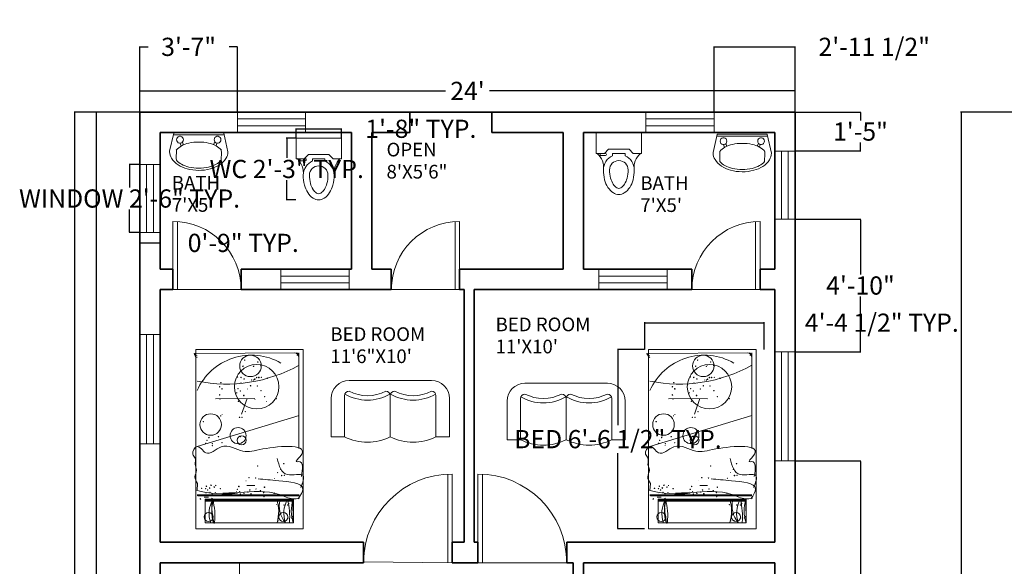
# Model space of a CAD drawing. Units: inches. Extents: x 125 to 976, y 231 to 853.
# Tile 11 of 16: x 125 to 557, y 613 to 853. Entities that reach past the tile are written whole.
import ezdxf

# ---------------------------------------------------------------- set-up
doc = ezdxf.new("R2010")
doc.units = ezdxf.units.IN
doc.header["$MEASUREMENT"] = 0
for name, color, linetype, lineweight in [('A-ANNO-DIMS', 2, 'Continuous', 18), ('A-AREA-IDEN', 7, 'Continuous', 18), ('A-DOOR', 3, 'Continuous', 18), ('A-FLOR-CASE', 32, 'Continuous', 18), ('A-FLOR-FIXT', 9, 'Continuous', 18), ('A-GLAZ', 4, 'Continuous', 18), ('A-WALL', 7, 'Continuous', 35), ('Furniture', 8, 'Continuous', 15)]:
    doc.layers.add(name, color=color, linetype=linetype, lineweight=lineweight)
doc.styles.get("Standard").update_dxf_attribs({"font": 'italic8.shx'})
doc.dimstyles.get("Standard").update_dxf_attribs({"dimtxt": 8, "dimasz": 0.18, "dimexe": 0.18, "dimexo": 0.0625, "dimgap": 0.09, "dimtad": 0, "dimtih": 1, "dimtoh": 1, "dimdec": 4, "dimzin": 0, "dimdsep": 46, "dimlunit": 3, "dimtxsty": 'Standard', "dimcen": 0.09, "dimclrt": 4, "dimadec": 0, "dimazin": 0, "dimtfac": 1, "dimtdec": 4, "dimtofl": 0, "dimtmove": 0, "dimatfit": 3, "dimfxl": 1, "dimtolj": 1, "dimtzin": 0, "dimarcsym": 0})

# ---------------------------------------------------------------- blocks, each defined once
blk = doc.blocks.new('*D3')
at = {"layer": 'A-ANNO-DIMS', "color": 0, "lineweight": -2, "transparency": 16777216}
for p, q in [((177.58, 812.17), (177.58, 821.62)), ((177.76, 821.44), (311.97, 821.44)), ((465.4, 821.44), (331.19, 821.44)), ((465.58, 812.17), (465.58, 821.62))]:
    blk.add_line(p, q, dxfattribs=at)
at = {"layer": 'A-ANNO-DIMS', "color": 0, "transparency": 16777216}
for points in [[(177.76, 821.47), (177.76, 821.41), (177.58, 821.44)], [(465.4, 821.47), (465.4, 821.41), (465.58, 821.44)]]:
    blk.add_solid(points, dxfattribs=at)
at = {"layer": 'Defpoints', "color": 0, "transparency": 16777216}
for p in [(465.58, 821.44), (177.58, 812.1), (465.58, 812.1)]:
    blk.add_point(p, dxfattribs=at)
at = {"layer": 'A-ANNO-DIMS', "color": 0, "transparency": 16777216, "insert": (321.58, 821.44), "char_height": 8, "attachment_point": 5}
blk.add_mtext("\\A1;24'", dxfattribs=at)
blk = doc.blocks.new('*D4')
at = {"layer": 'A-ANNO-DIMS', "color": 0, "lineweight": -2, "transparency": 16777216}
for p, q in [((177.52, 812.1), (158.26, 812.1)), ((158.44, 811.92), (158.44, 546.96)), ((158.44, 272.28), (158.44, 537.25)), ((177.52, 272.1), (158.26, 272.1))]:
    blk.add_line(p, q, dxfattribs=at)
at = {"layer": 'A-ANNO-DIMS', "color": 0, "transparency": 16777216}
for points in [[(158.41, 811.92), (158.47, 811.92), (158.44, 812.1)], [(158.41, 272.28), (158.47, 272.28), (158.44, 272.1)]]:
    blk.add_solid(points, dxfattribs=at)
at = {"layer": 'Defpoints', "color": 0, "transparency": 16777216}
for p in [(177.58, 812.1), (158.44, 272.1), (177.58, 272.1)]:
    blk.add_point(p, dxfattribs=at)
at = {"layer": 'A-ANNO-DIMS', "color": 0, "transparency": 16777216, "insert": (158.44, 542.1), "char_height": 8, "attachment_point": 5}
blk.add_mtext("\\A1;45'", dxfattribs=at)
blk = doc.blocks.new('BED-SINGLE')
for p, q in [((1.36, 0), (1.36, 78.74)), ((1.36, 78.74), (48.6, 78.74)), ((48.6, 78.74), (48.6, 0)), ((45.57, 77.25), (0.68, 77.02)), ((46.62, 76.32), (45.83, 76.32)), ((46.75, 35.25), (46.75, 77.26)), ((46.75, 35.25), (46.75, 75.28)), ((10.09, 57.07), (27.33, 57.29)), ((21.53, 50.36), (23.91, 57.3)), ((46.77, 49.81), (2, 36.21)), ((46.74, 50.11), (46.74, 35.53)), ((2.2, 19.89), (1.98, 16.84)), ((23.9, 19.06), (27.33, 19.06)), ((46.77, 14.92), (2, 14.9)), ((46.77, 14.62), (2, 14.6)), ((46.75, 14.47), (2.3, 14.45)), ((5.12, 13.84), (6.96, 13.84)), ((44.11, 12.79), (5.52, 12.79)), ((44.11, 12.66), (5.52, 12.66)), ((44.11, 12.36), (5.52, 12.36)), ((44.11, 12.07), (5.52, 12.07)), ((5.56, 2.64), (5.56, 12.97)), ((5.56, 12.97), (44.32, 12.97)), ((44.26, 2.65), (44.11, 12.79)), ((44.32, 12.97), (44.32, 2.64)), ((44.32, 2.64), (5.56, 2.64)), ((1.36, 0), (48.6, 0))]:
    blk.add_line(p, q)
for centre, radius in [((25.44, 71.55), 4.72), ((22.93, 74.08), 0.0787), ((28.17, 62.4), 9.76), ((22.09, 71.4), 0.118), ((26.78, 71.35), 0.118), ((27.34, 71.86), 0.0394), ((28.65, 73.29), 0.118), ((30.02, 71.69), 0.118), ((19.72, 66.71), 0.118), ((21.26, 66.47), 0.118), ((22.64, 65.78), 0.118), ((25.97, 65.38), 0.0394), ((26.83, 65.34), 0.118), ((27.33, 65.73), 0.118), ((28.16, 66.42), 0.118), ((29.11, 66.45), 0.118), ((30.23, 66.51), 0.0787), ((32.84, 66.14), 0.118), ((11.89, 62.39), 0.118), ((12.45, 64.21), 0.118), ((12.91, 61.47), 0.118), ((19.93, 61.53), 0.0787), ((21.3, 64.04), 0.0787), ((24.15, 61.41), 0.0394), ((25.46, 62.84), 0.118), ((28.4, 62.67), 0.0787), ((30.08, 60.69), 0.118), ((11.89, 58.82), 0.118), ((12.09, 56.97), 0.0787), ((19.37, 59.72), 0.0787), ((22.48, 58.54), 0.118), ((27.41, 56.76), 0.0394), ((31.66, 58.02), 0.0787), ((36.84, 57.2), 0.0787), ((20.18, 56), 0.118), ((32.59, 55.94), 0.0394), ((7.95, 45.79), 4.72), ((12.36, 49.61), 0.0787), ((12.97, 50.24), 0.0394), ((20.64, 48.94), 0.118), ((21.75, 49), 0.0787), ((23.12, 51.5), 0.0787), ((4.72, 47.06), 0.118), ((20, 40.91), 3.54), ((7.15, 40.05), 0.118), ((11.34, 40.44), 0.118), ((21.58, 38.87), 1.97), ((5.78, 37.54), 0.118), ((6.3, 38.84), 0.0787), ((8.67, 36.51), 0.0394), ((8.72, 37.38), 0.0787), ((12.92, 37.77), 0.0787), ((19.76, 37.58), 0.0394), ((28.63, 27.54), 0.0787), ((38.69, 26.11), 0.118), ((40.06, 28.61), 0.118), ((24.77, 22.46), 0.118), ((27.72, 22.29), 0.0787), ((36.01, 22.18), 0.0394), ((37.38, 24.68), 0.0394), ((39.15, 23.37), 0.118), ((40.26, 23.43), 0.0787), ((3.99, 17.75), 0.118), ((5.75, 17.64), 0.0787), ((6.1, 18.69), 0.118), ((7.26, 18.11), 0.0394), ((7.48, 17.87), 0.118), ((8.13, 19.13), 0.118), ((9.51, 18.3), 0.118), ((10.16, 19), 0.0787), ((12.17, 17.6), 0.118), ((19.68, 17.32), 0.118), ((20.33, 18.58), 0.118), ((23.46, 21.04), 0.0394), ((27.92, 17.51), 0.0787), ((31.59, 18.26), 0.118), ((3.44, 13.12), 0.118), ((5.89, 15.61), 0.0394), ((6.65, 17.04), 0.118), ((7.14, 14.65), 0.0394), ((7.68, 16.02), 0.0787), ((8.57, 13.26), 0.118), ((8.58, 15.39), 0.118), ((9.94, 15.76), 0.118), ((11.85, 14.52), 0.118), ((19.22, 16.39), 0.0394), ((20.71, 16.3), 0.0787), ((22.61, 15.56), 0.118), ((24.29, 16.17), 0.118), ((25.12, 17), 0.118), ((25.67, 15.35), 0.118), ((29.81, 16.72), 0.118), ((31.19, 15.9), 0.118), ((31.38, 14.05), 0.0787), ((35.87, 15.62), 0.118), ((36.87, 10.58), 0.0394), ((40.18, 10.43), 0.118), ((41.76, 10.43), 0.118), ((42.23, 11.05), 0.118), ((7.01, 5.19), 1.97), ((37.65, 4.55), 0.0394), ((39.85, 5.18), 1.97), ((41.9, 4.7), 0.0787), ((43.48, 4.7), 0.0787), ((43.95, 5.33), 0.0787), ((37.65, 3.45), 0.0394), ((39.23, 3.45), 0.0394), ((39.7, 4.08), 0.0394)]:
    blk.add_circle(centre, radius)
for centre, radius, start, end in [((1.8, 77.16), 1.13, 187.0311, 279.2977), ((2.15, 76.26), 1.02, 131.9337, 260.5378), ((25.86, 50.2), 26.08, 60.1506, 156.1931), ((44.78, 75.28), 1.97, 0, 90), ((45.57, 76.07), 1.18, 0, 90), ((14.92, 129.11), 65.53, 258.633, 299.0775), ((14.39, 67.77), 52.46, 255.8437, 275.7821), ((19.25, 6.76), 12.01, 149.8072, 199.9256), ((25.9, 7.71), 17.5, 163.1329, 196.7593), ((39.3, 10.2), 30.85, 175.6161, 194.8863), ((-19.02, 5.5), 28.83, 354.7074, 14.6885), ((19.98, 7.67), 17.85, 343.6634, 17.1743), ((49.46, 10.01), 11.36, 165.8396, 220.337), ((52.09, 6.75), 12.01, 149.8072, 199.9256), ((13.83, 5.48), 28.83, 354.7074, 14.6885), ((59.92, 7.95), 16.53, 163.0006, 198.6759)]:
    blk.add_arc(centre, radius, start, end)
for points, knots in [([(47.83, 23.01), (48.39, 26.23), (49.02, 29.87), (44.73, 29.28), (54.44, 37.77), (31.08, 35.83), (22.32, 32.61), (13.25, 38.92), (6.29, 30.55), (2.31, 38.17), (-0.92, 33.01), (1.74, 30.96), (0.68, 28.27), (2.31, 25.67), (0.37, 22.75), (1.58, 20.86), (2.2, 19.89)], [0, 0, 0, 0, 6.608381, 7.436978, 10.160479, 26.82811, 35.651646, 45.441607, 52.697614, 57.347481, 61.162366, 63.231685, 65.951856, 68.505046, 71.545852, 74.730692, 74.730692, 74.730692, 74.730692]), ([(47.57, 18.18), (48.41, 20.34), (50.37, 25.33), (39.55, 21.84), (38.02, 27.69), (37.18, 30.9)], [0, 0, 0, 0, 5.247261, 12.129135, 20.530793, 20.530793, 20.530793, 20.530793]), ([(46.4, 13.16), (47.43, 14.71), (50.88, 19.94), (37.54, 21.11), (31.56, 21.67), (28.88, 21.92)], [0, 0, 0, 0, 4.712342, 15.867179, 24.91455, 24.91455, 24.91455, 24.91455]), ([(13.24, 15.66), (15.6, 15.7), (23.87, 15.87), (34.62, 17.37), (42.93, 12.79), (46.01, 13.25), (47.01, 13.4)], [0, 0, 0, 0, 7.121262, 24.909491, 31.123221, 34.101394, 34.101394, 34.101394, 34.101394])]:
    blk.add_open_spline(points, degree=3, knots=knots)
for p in [(21.03, 60.57), (21.03, 40.49), (21.03, 15.28)]:
    blk.add_point(p)
blk = doc.blocks.new('WC')
for p, q in [((0, 27.17), (19.92, 27.17)), ((0, 27.17), (0, 18.11)), ((19.92, 27.17), (19.92, 18.11)), ((0, 18.11), (3.62, 18.11)), ((1.81, 18.11), (1.81, 17.21)), ((5.43, 19.92), (3.62, 18.11)), ((4.07, 18.11), (3.62, 18.11)), ((5.43, 19.92), (14.48, 19.92)), ((12.67, 18.11), (7.24, 18.11)), ((7.24, 18.11), (7.24, 17.09)), ((12.67, 18.11), (12.67, 17.09)), ((14.48, 19.92), (16.3, 18.11)), ((19.92, 18.11), (16.3, 18.11)), ((1.81, 17.21), (4.07, 17.21))]:
    blk.add_line(p, q)
for centre, radius, start, end in [((-4.9, 11.97), 8.15, 352.2011, 48.911), ((4.07, 17.66), 0.453, 270, 90), ((24.82, 11.97), 8.15, 131.089, 187.7989), ((9.96, 10.87), 6.79, 113.5782, 180), ((9.96, 10.87), 4.07, 0, 180), ((9.96, 10.87), 6.79, 0, 66.4218), ((20.49, 10.87), 17.33, 180, 194.5143), ((20.49, 10.87), 14.61, 180, 194.5142), ((-0.58, 10.87), 14.61, 345.4858, 360), ((-0.58, 10.87), 17.33, 345.4857, 360), ((15.3, 9.52), 11.96, 194.5143, 212.0054), ((15.3, 9.52), 9.24, 194.5143, 212.0054), ((12.02, 7.47), 5.38, 212.0054, 236.4659), ((7.9, 7.47), 5.38, 303.5341, 327.9946), ((4.62, 9.52), 9.24, 327.9946, 345.4857), ((4.62, 9.52), 11.96, 327.9946, 345.4857), ((12.02, 7.47), 8.09, 212.0054, 236.4659), ((9.96, 4.37), 4.36, 236.4659, 270), ((9.96, 4.37), 1.65, 236.466, 270), ((9.96, 4.37), 1.65, 270, 303.534), ((9.96, 4.37), 4.36, 270, 303.5341), ((7.9, 7.47), 8.09, 303.5341, 327.9946)]:
    blk.add_arc(centre, radius, start, end)
blk = doc.blocks.new('BASIN')
for p, q in [((0.01, 8.4), (1.8, 16.33)), ((1.8, 16.54), (23.8, 16.54)), ((1.8, 16.13), (1.8, 16.54)), ((23.8, 15.65), (1.8, 15.65)), ((3.17, 14), (3.08, 13.48)), ((3.08, 13.48), (3.17, 12.95)), ((3.42, 14.46), (3.17, 14)), ((3.81, 14.8), (3.42, 14.46)), ((4.29, 14.98), (3.81, 14.8)), ((4.81, 14.98), (4.29, 14.98)), ((5.29, 14.8), (4.81, 14.98)), ((5.68, 14.46), (5.29, 14.8)), ((5.93, 14), (5.68, 14.46)), ((6.02, 13.48), (5.93, 14)), ((5.93, 12.95), (6.02, 13.48)), ((19.66, 14), (19.58, 13.48)), ((19.58, 13.48), (19.66, 12.95)), ((19.92, 14.46), (19.66, 14)), ((20.31, 14.8), (19.92, 14.46)), ((20.79, 14.98), (20.31, 14.8)), ((21.3, 14.98), (20.79, 14.98)), ((21.79, 14.8), (21.3, 14.98)), ((22.18, 14.46), (21.79, 14.8)), ((22.43, 14), (22.18, 14.46)), ((22.52, 13.48), (22.43, 14)), ((22.43, 12.95), (22.52, 13.48)), ((23.8, 16.54), (23.8, 16.13)), ((25.59, 8.23), (23.8, 16.33)), ((2.96, 8.83), (2.87, 5.21)), ((2.97, 8.99), (2.96, 8.98)), ((2.96, 8.98), (2.96, 8.97)), ((2.96, 8.97), (2.96, 8.96)), ((2.96, 8.83), (2.96, 8.96)), ((3.07, 9.08), (2.97, 8.99)), ((3.17, 12.95), (3.42, 12.49)), ((3.42, 12.49), (3.81, 12.15)), ((3.81, 12.15), (4.29, 11.97)), ((4.29, 11.97), (4.81, 11.97)), ((4.57, 11.96), (5.02, 10.67)), ((4.81, 11.97), (5.29, 12.15)), ((5.29, 12.15), (5.68, 12.49)), ((5.63, 12.45), (6.09, 11.17)), ((5.68, 12.49), (5.93, 12.95)), ((19.87, 12.63), (19.34, 11.26)), ((19.66, 12.95), (19.92, 12.49)), ((19.92, 12.49), (20.31, 12.15)), ((20.31, 12.15), (20.79, 11.97)), ((20.73, 11.97), (20.41, 10.75)), ((20.79, 11.97), (21.3, 11.97)), ((21.3, 11.97), (21.79, 12.15)), ((21.79, 12.15), (22.18, 12.49)), ((22.18, 12.49), (22.43, 12.95)), ((22.76, 8.08), (22.65, 8.8)), ((2.87, 5.21), (3, 4.47)), ((22.54, 4.2), (22.57, 4.35)), ((22.6, 4.46), (22.76, 8.08)), ((3.05, 4.25), (3.05, 4.25))]:
    blk.add_line(p, q)
for centre, radius, start, end in [((8.91, 3.9), 7.83, 118.2302, 139.6822), ((11.35, -0.82), 13.14, 102.6999, 117.8694), ((12.88, -8.38), 20.85, 90.2298, 102.2344), ((12.72, -8.38), 20.85, 77.7656, 89.7702), ((14.25, -0.82), 13.14, 62.1306, 77.3001), ((16.68, 3.89), 7.83, 39.3299, 61.7657), ((5.18, 8.21), 5.18, 177.9266, 179.8113), ((5.16, 8.15), 5.16, 179.1785, 213.1413), ((8.98, 10.54), 9.66, 212.6461, 237.0936), ((8.91, 9.59), 7.83, 220.8964, 241.7723), ((16.69, 9.59), 7.83, 298.2281, 319.1983), ((16.64, 10.51), 9.66, 302.4413, 326.8887), ((20.44, 8.09), 5.16, 326.4084, 0.3713), ((20.42, 8.14), 5.18, 359.7541, 0.9471), ((11.42, 14.45), 14.27, 237.383, 254.6821), ((11.35, 14.31), 13.14, 242.1306, 257.3001), ((12.95, 20.75), 20.75, 255.1956, 269.4863), ((12.88, 21.87), 20.85, 257.7656, 269.7702), ((12.76, 20.75), 20.75, 270.0316, 284.3223), ((12.72, 21.87), 20.85, 270.2298, 282.2344), ((14.25, 14.31), 13.14, 282.6999, 297.8694), ((14.23, 14.44), 14.27, 284.841, 302.14)]:
    blk.add_arc(centre, radius, start, end)
blk = doc.blocks.new('LOVESEAT')
for p, q in [((44.1, 27.17, -27), (7.88, 27.17, -27)), ((0, 19.29, -27), (0, 2.36, -27)), ((5.91, 20.47, -27), (5.91, 2.36, -27)), ((5.91, 2.36, -27), (5.91, 20.47, -27)), ((5.91, 20.47, -27), (5.91, 2.36, -27)), ((25.99, 2.36, -27), (25.99, 20.47, -27)), ((25.99, 20.47, -27), (25.99, 2.36, -27)), ((46.07, 20.47, -27), (46.07, 2.36, -27)), ((51.97, 2.36, -27), (51.97, 19.29, -27)), ((0, 2.36, -27), (5.91, 2.36, -27)), ((51.97, 2.36, -27), (46.07, 2.36, -27))]:
    blk.add_line(p, q)
for centre, radius, start, end in [((7.88, 19.29, -27), 7.87, 90, 180), ((44.1, 19.29, -27), 7.87, 0, 90), ((7.88, 20.47, -27), 1.97, 90, 180), ((15.95, 38, -27), 17.53, 242.5861, 297.4139), ((24.02, 20.47, -27), 1.97, 0, 90), ((27.96, 20.47, -27), 1.97, 90, 180), ((36.03, 38, -27), 17.53, 242.5861, 297.4139), ((44.1, 20.47, -27), 1.97, 0, 90), ((15.95, 38, -27), 19.5, 239.4911, 300.5089), ((36.03, 38, -27), 19.5, 239.4911, 300.5089), ((15.95, 22.51, -27), 22.51, 243.519, 296.481), ((36.03, 22.51, -27), 22.51, 243.519, 296.481)]:
    blk.add_arc(centre, radius, start, end)
blk = doc.blocks.new('WINDOW-48IN')
for p, q in [((0, 0), (0, 48)), ((0, 48), (9, 48)), ((3, 0), (3, 48)), ((6, 0), (6, 48)), ((9, 48), (9, 0)), ((9, 0), (0, 0))]:
    blk.add_line(p, q)
blk = doc.blocks.new('WINDOW-30IN')
for p, q in [((0, 0), (0, 9)), ((0, 9), (30, 9)), ((30, 9), (30, 0)), ((30, 6), (0, 6)), ((30, 3), (0, 3)), ((30, 0), (0, 0))]:
    blk.add_line(p, q)
blk = doc.blocks.new('DOOR-39IN-LH')
for p, q in [((-2, 0), (-2, 38.95)), ((0, 0), (0, 39)), ((-39, 0.34), (0, 0))]:
    blk.add_line(p, q)
blk.add_arc((0, 0), 39, 90, 179.5065)
blk = doc.blocks.new('DOOR-39IN-RH')
for p, q in [((0, 39), (0, 0)), ((2, 38.95), (2, 0)), ((0, 0), (39, 0))]:
    blk.add_line(p, q)
blk.add_arc((0, 0), 39, 0, 90)
blk = doc.blocks.new('DOOR-30IN')
for p, q in [((-2, 29.93), (-2, 0)), ((0, 30), (0, 0)), ((0, 0), (-30, 0))]:
    blk.add_line(p, q)
blk.add_arc((0, 0), 30, 90, 180)
blk = doc.blocks.new('*D26')
at = {"layer": 'A-ANNO-DIMS', "color": 0, "lineweight": -2, "transparency": 16777216}
for p, q in [((177.52, 789.16), (172.9, 789.16)), ((173.08, 788.98), (173.08, 779.01)), ((173.08, 759.34), (173.08, 769.3)), ((177.52, 759.16), (172.9, 759.16))]:
    blk.add_line(p, q, dxfattribs=at)
at = {"layer": 'A-ANNO-DIMS', "color": 0, "transparency": 16777216}
for points in [[(173.05, 788.98), (173.11, 788.98), (173.08, 789.16)], [(173.05, 759.34), (173.11, 759.34), (173.08, 759.16)]]:
    blk.add_solid(points, dxfattribs=at)
at = {"layer": 'Defpoints', "color": 0, "transparency": 16777216}
for p in [(177.58, 789.16), (173.08, 759.16), (177.58, 759.16)]:
    blk.add_point(p, dxfattribs=at)
at = {"layer": 'A-ANNO-DIMS', "color": 4, "transparency": 16777216, "insert": (173.08, 774.16), "char_height": 8, "attachment_point": 5}
blk.add_mtext('\\A1;WINDOW 2\'-6" TYP.', dxfattribs=at)
blk = doc.blocks.new('*D27')
at = {"layer": 'A-ANNO-DIMS', "color": 0, "lineweight": -2, "transparency": 16777216}
for p, q in [((177.58, 759.09), (177.58, 754.48)), ((186.58, 759.09), (186.58, 754.48)), ((177.76, 754.66), (186.4, 754.66)), ((186.58, 754.66), (186.76, 754.66))]:
    blk.add_line(p, q, dxfattribs=at)
at = {"layer": 'A-ANNO-DIMS', "color": 0, "transparency": 16777216}
for points in [[(177.76, 754.69), (177.76, 754.63), (177.58, 754.66)], [(186.4, 754.69), (186.4, 754.63), (186.58, 754.66)]]:
    blk.add_solid(points, dxfattribs=at)
at = {"layer": 'Defpoints', "color": 0, "transparency": 16777216}
for p in [(177.58, 759.16), (186.58, 759.16), (186.58, 754.66)]:
    blk.add_point(p, dxfattribs=at)
at = {"layer": 'A-ANNO-DIMS', "color": 4, "transparency": 16777216, "insert": (223.04, 754.66), "char_height": 8, "attachment_point": 5}
blk.add_mtext('\\A1;0\'-9" TYP.', dxfattribs=at)
blk = doc.blocks.new('*D30')
at = {"layer": 'A-ANNO-DIMS', "color": 0, "lineweight": -2, "transparency": 16777216}
for p, q in [((399.43, 707.79), (387.5, 707.79)), ((387.68, 707.61), (387.68, 674.6)), ((387.68, 629.23), (387.68, 662.23)), ((399.43, 629.05), (387.5, 629.05))]:
    blk.add_line(p, q, dxfattribs=at)
at = {"layer": 'A-ANNO-DIMS', "color": 0, "transparency": 16777216}
for points in [[(387.65, 707.61), (387.71, 707.61), (387.68, 707.79)], [(387.65, 629.23), (387.71, 629.23), (387.68, 629.05)]]:
    blk.add_solid(points, dxfattribs=at)
at = {"layer": 'Defpoints', "color": 0, "transparency": 16777216}
for p in [(387.68, 707.79), (399.49, 707.79), (399.49, 629.05)]:
    blk.add_point(p, dxfattribs=at)
at = {"layer": 'A-ANNO-DIMS', "color": 4, "transparency": 16777216, "insert": (387.68, 668.42), "char_height": 8, "attachment_point": 5}
blk.add_mtext('\\A1;BED 6\'-6 1/2" TYP.', dxfattribs=at)
blk = doc.blocks.new('*D31')
at = {"layer": 'A-ANNO-DIMS', "color": 0, "lineweight": -2, "transparency": 16777216}
for p, q in [((399.49, 707.85), (399.49, 719.78)), ((399.67, 719.6), (451.78, 719.6)), ((451.96, 707.85), (451.96, 719.78)), ((451.96, 719.6), (452.14, 719.6))]:
    blk.add_line(p, q, dxfattribs=at)
at = {"layer": 'A-ANNO-DIMS', "color": 0, "transparency": 16777216}
for points in [[(399.67, 719.63), (399.67, 719.57), (399.49, 719.6)], [(451.78, 719.63), (451.78, 719.57), (451.96, 719.6)]]:
    blk.add_solid(points, dxfattribs=at)
at = {"layer": 'Defpoints', "color": 0, "transparency": 16777216}
for p in [(451.96, 719.6), (399.49, 707.79), (451.96, 707.79)]:
    blk.add_point(p, dxfattribs=at)
at = {"layer": 'A-ANNO-DIMS', "color": 4, "transparency": 16777216, "insert": (503.66, 719.6), "char_height": 8, "attachment_point": 5}
blk.add_mtext('\\A1;4\'-4 1/2" TYP.', dxfattribs=at)
blk = doc.blocks.new('*D32')
at = {"layer": 'A-ANNO-DIMS', "color": 0, "lineweight": -2, "transparency": 16777216}
for p, q in [((246.17, 800.72), (241.97, 800.72)), ((242.15, 800.54), (242.15, 791.99)), ((242.15, 773.74), (242.15, 782.29)), ((246.17, 773.56), (241.97, 773.56))]:
    blk.add_line(p, q, dxfattribs=at)
at = {"layer": 'A-ANNO-DIMS', "color": 0, "transparency": 16777216}
for points in [[(242.12, 800.54), (242.18, 800.54), (242.15, 800.72)], [(242.12, 773.74), (242.18, 773.74), (242.15, 773.56)]]:
    blk.add_solid(points, dxfattribs=at)
at = {"layer": 'Defpoints', "color": 0, "transparency": 16777216}
for p in [(242.15, 800.72), (246.23, 800.72), (246.23, 773.56)]:
    blk.add_point(p, dxfattribs=at)
at = {"layer": 'A-ANNO-DIMS', "color": 4, "transparency": 16777216, "insert": (242.15, 787.14), "char_height": 8, "attachment_point": 5}
blk.add_mtext('\\A1;WC 2\'-3" TYP.', dxfattribs=at)
blk = doc.blocks.new('*D33')
at = {"layer": 'A-ANNO-DIMS', "color": 0, "lineweight": -2, "transparency": 16777216}
for p, q in [((246.23, 800.79), (246.23, 804.98)), ((266.15, 800.79), (266.15, 804.98)), ((246.41, 804.8), (265.97, 804.8)), ((266.15, 804.8), (266.33, 804.8))]:
    blk.add_line(p, q, dxfattribs=at)
at = {"layer": 'A-ANNO-DIMS', "color": 0, "transparency": 16777216}
for points in [[(246.41, 804.83), (246.41, 804.77), (246.23, 804.8)], [(265.97, 804.83), (265.97, 804.77), (266.15, 804.8)]]:
    blk.add_solid(points, dxfattribs=at)
at = {"layer": 'Defpoints', "color": 0, "transparency": 16777216}
for p in [(246.23, 800.72), (266.15, 804.8), (266.15, 800.72)]:
    blk.add_point(p, dxfattribs=at)
at = {"layer": 'A-ANNO-DIMS', "color": 4, "transparency": 16777216, "insert": (301.09, 804.8), "char_height": 8, "attachment_point": 5}
blk.add_mtext('\\A1;1\'-8" TYP.', dxfattribs=at)
blk = doc.blocks.new('*D56')
at = {"layer": 'A-ANNO-DIMS', "color": 0, "lineweight": -2, "transparency": 16777216}
for p, q in [((177.52, 812.1), (148.7, 812.1)), ((148.88, 811.92), (148.88, 575.46)), ((148.88, 329.28), (148.88, 565.75)), ((186.52, 329.1), (148.7, 329.1))]:
    blk.add_line(p, q, dxfattribs=at)
at = {"layer": 'A-ANNO-DIMS', "color": 0, "transparency": 16777216}
for points in [[(148.85, 811.92), (148.91, 811.92), (148.88, 812.1)], [(148.85, 329.28), (148.91, 329.28), (148.88, 329.1)]]:
    blk.add_solid(points, dxfattribs=at)
at = {"layer": 'Defpoints', "color": 0, "transparency": 16777216}
for p in [(148.88, 812.1), (177.58, 812.1), (186.58, 329.1)]:
    blk.add_point(p, dxfattribs=at)
at = {"layer": 'A-ANNO-DIMS', "color": 4, "transparency": 16777216, "insert": (148.88, 570.6), "char_height": 8, "attachment_point": 5}
blk.add_mtext('\\A1;40\'-3"', dxfattribs=at)
blk = doc.blocks.new('*D57')
at = {"layer": 'A-ANNO-DIMS', "color": 0, "lineweight": -2, "transparency": 16777216}
for p, q in [((567.13, 812.1), (538.31, 812.1)), ((538.49, 811.92), (538.49, 575.46)), ((538.49, 329.28), (538.49, 565.75)), ((576.13, 329.1), (538.31, 329.1))]:
    blk.add_line(p, q, dxfattribs=at)
at = {"layer": 'A-ANNO-DIMS', "color": 0, "transparency": 16777216}
for points in [[(538.46, 811.92), (538.52, 811.92), (538.49, 812.1)], [(538.46, 329.28), (538.52, 329.28), (538.49, 329.1)]]:
    blk.add_solid(points, dxfattribs=at)
at = {"layer": 'Defpoints', "color": 0, "transparency": 16777216}
for p in [(538.49, 812.1), (567.19, 812.1), (576.19, 329.1)]:
    blk.add_point(p, dxfattribs=at)
at = {"layer": 'A-ANNO-DIMS', "color": 4, "transparency": 16777216, "insert": (538.49, 570.6), "char_height": 8, "attachment_point": 5}
blk.add_mtext('\\A1;40\'-3"', dxfattribs=at)
blk = doc.blocks.new('*D64')
at = {"layer": 'A-ANNO-DIMS', "color": 0, "lineweight": -2, "transparency": 16777216}
for p, q in [((465.64, 658.83), (494.46, 658.83)), ((494.28, 658.65), (494.28, 561.16)), ((494.28, 451.31), (494.28, 548.79)), ((465.64, 451.13), (494.46, 451.13))]:
    blk.add_line(p, q, dxfattribs=at)
at = {"layer": 'A-ANNO-DIMS', "color": 0, "transparency": 16777216}
for points in [[(494.25, 658.65), (494.31, 658.65), (494.28, 658.83)], [(494.25, 451.31), (494.31, 451.31), (494.28, 451.13)]]:
    blk.add_solid(points, dxfattribs=at)
at = {"layer": 'Defpoints', "color": 0, "transparency": 16777216}
for p in [(465.58, 658.83), (494.28, 658.83), (465.58, 451.13)]:
    blk.add_point(p, dxfattribs=at)
at = {"layer": 'A-ANNO-DIMS', "color": 4, "transparency": 16777216, "insert": (494.28, 554.98), "char_height": 8, "attachment_point": 5}
blk.add_mtext('\\A1;17\'-3 1/2"', dxfattribs=at)
blk = doc.blocks.new('*D65')
at = {"layer": 'A-ANNO-DIMS', "color": 0, "lineweight": -2, "transparency": 16777216}
for p, q in [((465.64, 765.04), (494.46, 765.04)), ((494.28, 764.86), (494.28, 740.78)), ((494.28, 707.01), (494.28, 731.08)), ((465.64, 706.83), (494.46, 706.83))]:
    blk.add_line(p, q, dxfattribs=at)
at = {"layer": 'A-ANNO-DIMS', "color": 0, "transparency": 16777216}
for points in [[(494.25, 764.86), (494.31, 764.86), (494.28, 765.04)], [(494.25, 707.01), (494.31, 707.01), (494.28, 706.83)]]:
    blk.add_solid(points, dxfattribs=at)
at = {"layer": 'Defpoints', "color": 0, "transparency": 16777216}
for p in [(465.58, 765.04), (494.28, 765.04), (465.58, 706.83)]:
    blk.add_point(p, dxfattribs=at)
at = {"layer": 'A-ANNO-DIMS', "color": 4, "transparency": 16777216, "insert": (494.28, 735.93), "char_height": 8, "attachment_point": 5}
blk.add_mtext('\\A1;4\'-10"', dxfattribs=at)
blk = doc.blocks.new('*D66')
at = {"layer": 'A-ANNO-DIMS', "color": 0, "lineweight": -2, "transparency": 16777216}
for p, q in [((465.64, 812.1), (494.46, 812.1)), ((494.28, 811.92), (494.28, 808.42)), ((494.28, 795.22), (494.28, 798.72)), ((465.64, 795.04), (494.46, 795.04))]:
    blk.add_line(p, q, dxfattribs=at)
at = {"layer": 'A-ANNO-DIMS', "color": 0, "transparency": 16777216}
for points in [[(494.25, 811.92), (494.31, 811.92), (494.28, 812.1)], [(494.25, 795.22), (494.31, 795.22), (494.28, 795.04)]]:
    blk.add_solid(points, dxfattribs=at)
at = {"layer": 'Defpoints', "color": 0, "transparency": 16777216}
for p in [(465.58, 812.1), (494.28, 812.1), (465.58, 795.04)]:
    blk.add_point(p, dxfattribs=at)
at = {"layer": 'A-ANNO-DIMS', "color": 4, "transparency": 16777216, "insert": (494.28, 803.57), "char_height": 8, "attachment_point": 5}
blk.add_mtext('\\A1;1\'-5"', dxfattribs=at)
blk = doc.blocks.new('*D67')
at = {"layer": 'A-ANNO-DIMS', "color": 0, "lineweight": -2, "transparency": 16777216}
for p, q in [((177.58, 812.17), (177.58, 840.98)), ((177.76, 840.8), (181.21, 840.8)), ((220.27, 840.8), (216.82, 840.8)), ((220.45, 812.17), (220.45, 840.98))]:
    blk.add_line(p, q, dxfattribs=at)
at = {"layer": 'A-ANNO-DIMS', "color": 0, "transparency": 16777216}
for points in [[(177.76, 840.83), (177.76, 840.77), (177.58, 840.8)], [(220.27, 840.83), (220.27, 840.77), (220.45, 840.8)]]:
    blk.add_solid(points, dxfattribs=at)
at = {"layer": 'Defpoints', "color": 0, "transparency": 16777216}
for p in [(220.45, 840.8), (177.58, 812.1), (220.45, 812.1)]:
    blk.add_point(p, dxfattribs=at)
at = {"layer": 'A-ANNO-DIMS', "color": 4, "transparency": 16777216, "insert": (199.02, 840.8), "char_height": 8, "attachment_point": 5}
blk.add_mtext('\\A1;3\'-7"', dxfattribs=at)
blk = doc.blocks.new('*D68')
at = {"layer": 'A-ANNO-DIMS', "color": 0, "lineweight": -2, "transparency": 16777216}
for p, q in [((429.95, 812.17), (429.95, 840.98)), ((430.13, 840.8), (465.4, 840.8)), ((465.58, 812.17), (465.58, 840.98)), ((465.58, 840.8), (465.76, 840.8))]:
    blk.add_line(p, q, dxfattribs=at)
at = {"layer": 'A-ANNO-DIMS', "color": 0, "transparency": 16777216}
for points in [[(430.13, 840.83), (430.13, 840.77), (429.95, 840.8)], [(465.4, 840.83), (465.4, 840.77), (465.58, 840.8)]]:
    blk.add_solid(points, dxfattribs=at)
at = {"layer": 'Defpoints', "color": 0, "transparency": 16777216}
for p in [(465.58, 840.8), (429.95, 812.1), (465.58, 812.1)]:
    blk.add_point(p, dxfattribs=at)
at = {"layer": 'A-ANNO-DIMS', "color": 4, "transparency": 16777216, "insert": (500.33, 840.8), "char_height": 8, "attachment_point": 5}
blk.add_mtext('\\A1;2\'-11 1/2"', dxfattribs=at)

msp = doc.modelspace()

# ---------------------------------------------------------------- linework, layer by layer
at = {"layer": 'A-FLOR-CASE'}
msp.add_line((221.33932, 535.92817), (221.33932, 614.10475), dxfattribs=at)
at = {"layer": 'A-WALL'}
for p, q in [((296.24923, 812.10475), (296.24923, 803.10475)), ((332.24923, 812.10475), (332.24923, 803.10475)), ((186.5792, 803.10475), (186.5792, 743.10475)), ((270.5792, 803.10475), (186.5792, 803.10475)), ((270.5792, 803.10475), (270.5792, 743.10475)), ((279.5792, 803.10475), (279.5792, 743.10475)), ((296.24923, 803.10475), (279.5792, 803.10475)), ((363.5792, 803.10475), (332.24923, 803.10475)), ((363.5792, 743.10475), (363.5792, 803.10475)), ((456.5792, 803.10475), (372.5792, 803.10475)), ((372.5792, 743.10475), (372.5792, 803.10475)), ((456.5792, 743.10475), (456.5792, 803.10475)), ((192.12733, 743.10475), (186.5792, 743.10475)), ((192.12733, 734.10475), (192.12733, 743.10475)), ((270.5792, 743.10475), (222.12733, 743.10475)), ((222.12733, 734.10475), (222.12733, 743.10475)), ((288.11104, 743.10475), (279.5792, 743.10475)), ((288.11104, 734.10475), (288.11104, 743.10475)), ((363.5792, 743.10475), (318.11104, 743.10475)), ((318.11104, 734.10475), (318.11104, 743.10475)), ((318.11104, 743.10475), (318.11104, 734.10475)), ((420.21882, 743.10475), (372.5792, 743.10475)), ((420.21882, 743.10475), (420.21882, 734.10475)), ((456.5792, 743.10475), (450.21882, 743.10475)), ((450.21882, 743.10475), (450.21882, 734.10475)), ((450.21882, 743.10475), (450.21882, 734.10475)), ((186.5792, 734.10475), (186.5792, 623.10475)), ((192.12733, 734.10475), (186.5792, 734.10475)), ((288.11104, 734.10475), (222.12733, 734.10475)), ((320.0792, 734.10475), (318.11104, 734.10475)), ((320.0792, 734.10475), (320.0792, 623.10475)), ((324.5792, 734.10475), (324.5792, 623.10475)), ((420.21882, 734.10475), (324.5792, 734.10475)), ((456.5792, 734.10475), (450.21882, 734.10475)), ((456.5792, 623.10475), (456.5792, 734.10475)), ((186.5792, 623.10475), (275.88045, 623.10475)), ((275.88045, 614.10475), (275.88045, 623.10475)), ((314.88045, 614.10475), (314.88045, 623.10475)), ((314.88045, 623.10475), (320.0792, 623.10475)), ((314.88045, 614.10475), (314.88045, 623.10475)), ((324.5792, 623.10475), (326.20254, 623.10475)), ((326.20254, 614.10475), (326.20254, 623.10475)), ((326.20254, 623.10475), (326.20254, 614.10475)), ((365.20254, 614.10475), (365.20254, 623.10475)), ((365.20254, 623.10475), (456.5792, 623.10475)), ((186.5792, 614.10475), (186.5792, 503.10475)), ((275.88045, 614.10475), (186.5792, 614.10475)), ((324.5792, 614.10475), (314.88045, 614.10475)), ((326.20254, 614.10475), (324.5792, 614.10475)), ((368.0792, 614.10475), (365.20254, 614.10475)), ((368.0792, 614.10475), (368.0792, 503.10475)), ((456.5792, 614.10475), (372.5792, 614.10475)), ((372.5792, 614.10475), (372.5792, 503.10475)), ((456.5792, 503.10475), (456.5792, 614.10475))]:
    msp.add_line(p, q, dxfattribs=at)
msp.add_lwpolyline([(177.5792, 272.10475), (465.5792, 272.10475), (465.5792, 812.10475), (177.5792, 812.10475)], close=True, dxfattribs=at)

# ---------------------------------------------------------------- block references
at = {"layer": 'A-DOOR', "extrusion": (0, 0, -1), "zscale": -1}
msp.add_blockref('DOOR-30IN', (-192.12733, 734.10475), dxfattribs=at)
at = {"layer": 'A-DOOR'}
for name, p in [('DOOR-30IN', (318.11104, 734.10475)), ('DOOR-30IN', (450.21882, 734.10475)), ('DOOR-39IN-LH', (314.88045, 614.10475)), ('DOOR-39IN-RH', (326.20254, 614.10475))]:
    msp.add_blockref(name, p, dxfattribs=at)
at = {"layer": 'A-FLOR-FIXT'}
for name, p in [('BASIN', (190.69, 786.51)), ('WC', (246.23365, 773.55779)), ('WC', (378.14, 775.87)), ('BASIN', (429.53981, 785.91375))]:
    msp.add_blockref(name, p, dxfattribs=at)
at = {"layer": 'A-GLAZ'}
for name, p in [('WINDOW-30IN', (220.45702, 803.1)), ('WINDOW-30IN', (399.95826, 803.1)), ('WINDOW-30IN', (239.57681, 734.1)), ('WINDOW-30IN', (379.29823, 734.1)), ('WINDOW-48IN', (177.57633, 666.40706)), ('WINDOW-48IN', (456.57633, 658.82339))]:
    msp.add_blockref(name, p, dxfattribs=at)
for p, rotation in [((456.57445, 795.03164), 270.0000000000005), ((177.57445, 789.15144), 270.0000000000001)]:
    msp.add_blockref('WINDOW-30IN', p, dxfattribs=dict(at, rotation=rotation))
at = {"layer": 'Furniture'}
for name, p in [('BED-SINGLE', (200.78, 629.05)), ('BED-SINGLE', (399.77711, 629.05)), ('LOVESEAT', (261.67015, 667.04447)), ('LOVESEAT', (338.95918, 665.80557))]:
    msp.add_blockref(name, p, dxfattribs=at)

# ---------------------------------------------------------------- texts
at = {"layer": 'A-AREA-IDEN'}
for s, p in [('OPEN', (286.00704, 792.65826)), ('8\'X5\'6"', (286.00704, 782.94397)), ('BATH', (191.64507, 778.05433)), ('BATH', (397.5437, 777.95704)), ("7'X5'", (191.64507, 768.34004)), ("7'X5'", (397.5437, 768.24275)), ('BED ROOM', (333.94404, 715.83249)), ('BED ROOM', (261.32664, 711.56438)), ("11'X10'", (333.94404, 706.1182)), ('11\'6"X10\'', (261.32664, 701.85009))]:
    msp.add_text(s, height=6, dxfattribs=at).set_placement(p)

# ---------------------------------------------------------------- dimensions: what is measured, and where the dimension line sits
at = {"layer": 'A-ANNO-DIMS'}
for base, p1, p2, override, picture, middle in [((465.5792, 840.80475), (429.95423, 812.10475), (465.5792, 812.10475), {"dimdec": 1, "dimlfac": 1, "dimrnd": 0, "dimzin": 1, "dimdsep": 46, "dimlunit": 4, "dimfrac": 2}, '*D68', (500.32539, 840.80475)), ((220.453, 840.80475), (177.5792, 812.10475), (220.453, 812.10475), {"dimdec": 1, "dimlfac": 1, "dimrnd": 0, "dimzin": 1, "dimdsep": 46, "dimlunit": 4, "dimfrac": 2}, '*D67', (199.0161, 840.80475)), ((465.5792, 821.43521), (177.5792, 812.10475), (465.5792, 812.10475), {"dimclrd": 0, "dimclre": 0, "dimclrt": 0}, '*D3', (321.5792, 821.43521))]:
    dim = msp.add_linear_dim(base=base, p1=p1, p2=p2, dimstyle='Standard', override=override, dxfattribs=at)
    dim.commit()
    dim.dimension.update_dxf_attribs({"geometry": picture, "text_midpoint": middle})
for base, p1, p2, picture, middle in [((266.15098, 804.79975), (246.22976, 800.72496), (266.15098, 800.72496), '*D33', (301.08765, 804.79975)), ((186.5792, 754.65547), (177.5792, 759.15547), (186.5792, 759.15547), '*D27', (223.03967, 754.65547)), ((451.95954, 719.60059), (399.49239, 707.78959), (451.95954, 707.78959), '*D31', (503.65811, 719.60059))]:
    dim = msp.add_linear_dim(base=base, p1=p1, p2=p2, text='<> TYP.', dimstyle='Standard', override={"dimdec": 1, "dimlfac": 1, "dimrnd": 0, "dimzin": 1, "dimdsep": 46, "dimlunit": 4, "dimfrac": 2}, dxfattribs=at)
    dim.commit()
    dim.dimension.update_dxf_attribs({"geometry": picture, "text_midpoint": middle})
for base, p1, p2, override, picture, middle in [((148.8792, 812.10475), (186.5792, 329.10475), (177.5792, 812.10475), {"dimdec": 1, "dimlfac": 1, "dimrnd": 0, "dimzin": 1, "dimdsep": 46, "dimlunit": 4, "dimfrac": 2}, '*D56', (148.8792, 570.60475)), ((158.44384, 272.10475), (177.5792, 812.10475), (177.5792, 272.10475), {"dimclrd": 0, "dimclre": 0, "dimclrt": 0}, '*D4', (158.44384, 542.10475)), ((494.2792, 812.10475), (465.5792, 795.03566), (465.5792, 812.10475), {"dimdec": 1, "dimlfac": 1, "dimrnd": 0, "dimzin": 1, "dimdsep": 46, "dimlunit": 4, "dimfrac": 2}, '*D66', (494.2792, 803.5702)), ((538.49287, 812.10475), (576.19287, 329.10475), (567.19287, 812.10475), {"dimdec": 1, "dimlfac": 1, "dimrnd": 0, "dimzin": 1, "dimdsep": 46, "dimlunit": 4, "dimfrac": 2}, '*D57', (538.49287, 570.60475)), ((494.2792, 765.03566), (465.5792, 706.82838), (465.5792, 765.03566), {"dimdec": 1, "dimlfac": 1, "dimrnd": 0, "dimzin": 1, "dimdsep": 46, "dimlunit": 4, "dimfrac": 2}, '*D65', (494.2792, 735.93202)), ((494.2792, 658.82838), (465.5792, 451.12515), (465.5792, 658.82838), {"dimdec": 1, "dimlfac": 1, "dimrnd": 0, "dimzin": 1, "dimdsep": 46, "dimlunit": 4, "dimfrac": 2}, '*D64', (494.2792, 554.97677))]:
    dim = msp.add_linear_dim(base=base, p1=p1, p2=p2, angle=90, dimstyle='Standard', override=override, dxfattribs=at)
    dim.commit()
    dim.dimension.update_dxf_attribs({"geometry": picture, "text_midpoint": middle})
for base, p1, p2, angle, text, picture, middle in [((242.15496, 800.72496), (246.22976, 773.55966), (246.22976, 800.72496), 90, 'WC <> TYP.', '*D32', (242.15496, 787.14231)), ((173.0792, 759.15547), (177.5792, 789.15547), (177.5792, 759.15547), 270, 'WINDOW <> TYP.', '*D26', (173.0792, 774.15547)), ((387.68139, 707.78959), (399.49239, 629.04959), (399.49239, 707.78959), 90, 'BED <> TYP.', '*D30', (387.68139, 668.41959))]:
    dim = msp.add_linear_dim(base=base, p1=p1, p2=p2, angle=angle, text=text, dimstyle='Standard', override={"dimdec": 1, "dimlfac": 1, "dimrnd": 0, "dimzin": 1, "dimdsep": 46, "dimlunit": 4, "dimfrac": 2}, dxfattribs=at)
    dim.commit()
    dim.dimension.update_dxf_attribs({"geometry": picture, "text_midpoint": middle})

doc.saveas('drawing.dxf')
